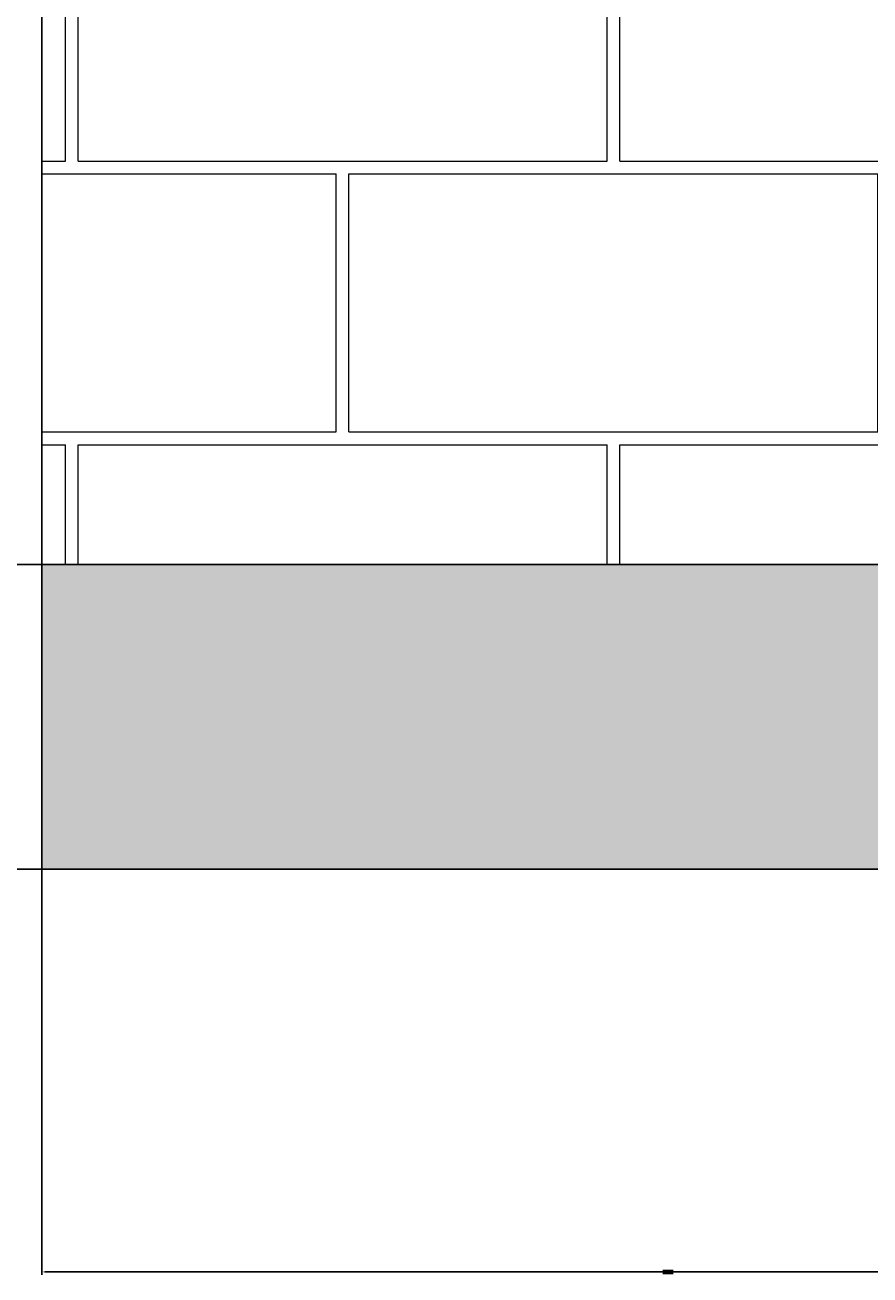
# Model space of a CAD drawing. Units: inches. Extents: x -128 to 854, y -395 to 398.
# Tile 52 of 61: x 417 to 467, y -395 to -322. Entities that reach past the tile are written whole.
import ezdxf

# ---------------------------------------------------------------- set-up
doc = ezdxf.new("R2010")
doc.units = ezdxf.units.IN
doc.header["$MEASUREMENT"] = 0
for name, color, linetype, lineweight in [('A-ANNO-DIMS', 2, 'Continuous', 18), ('A-ELEV', 3, 'Continuous', 25), ('A-ELEV-PATT', 8, 'Continuous', 13), ('C-GRAD', 7, 'Continuous', 25)]:
    doc.layers.add(name, color=color, linetype=linetype, lineweight=lineweight)
doc.styles.get("Standard").update_dxf_attribs({"font": 'arial.ttf'})
doc.dimstyles.get("Standard").update_dxf_attribs({"dimtxt": 0.18, "dimasz": 0.18, "dimexe": 0.18, "dimexo": 0.0625, "dimgap": 0.09, "dimtad": 0, "dimtih": 1, "dimtoh": 1, "dimdec": 1, "dimzin": 0, "dimdsep": 46, "dimlunit": 4, "dimtxsty": 'Standard', "dimcen": 0.09, "dimclrd": 1, "dimclre": 2, "dimclrt": 6, "dimadec": 0, "dimazin": 0, "dimtfac": 1, "dimtdec": 1, "dimtofl": 0, "dimtmove": 0, "dimatfit": 3, "dimfxl": 1, "dimtfill": 2, "dimtfillclr": 3, "dimtolj": 1, "dimtzin": 0, "dimarcsym": 0})

# ---------------------------------------------------------------- blocks, each defined once
blk = doc.blocks.new('*D134')
at = {"layer": 'A-ANNO-DIMS', "color": 2, "lineweight": -2, "transparency": 16777216}
for p, q in [((418.217, -191.476), (346.3, -191.476)), ((418.217, -371.476), (346.3, -371.476))]:
    blk.add_line(p, q, dxfattribs=at)
at = {"layer": 'A-ANNO-DIMS', "color": 1, "lineweight": -2, "transparency": 16777216}
for p, q in [((346.48, -191.656), (346.48, -281.295)), ((346.48, -371.296), (346.48, -281.658))]:
    blk.add_line(p, q, dxfattribs=at)
at = {"layer": 'A-ANNO-DIMS', "color": 1, "transparency": 16777216}
for points in [[(346.45, -191.656), (346.51, -191.656), (346.48, -191.476)], [(346.45, -371.296), (346.51, -371.296), (346.48, -371.476)]]:
    blk.add_solid(points, dxfattribs=at)
at = {"layer": 'Defpoints', "color": 0, "transparency": 16777216}
for p in [(346.48, -191.476), (418.28, -191.476), (418.28, -371.476)]:
    blk.add_point(p, dxfattribs=at)
at = {"layer": 'A-ANNO-DIMS', "color": 6, "transparency": 16777216, "insert": (346.48, -281.476), "char_height": 0.18, "attachment_point": 5, "bg_fill": 1, "box_fill_scale": 1.25, "bg_fill_color": 3, "bg_fill_transparency": 0}
blk.add_mtext('\\A1;15\'-0"', dxfattribs=at)
blk = doc.blocks.new('*D135')
at = {"layer": 'A-ANNO-DIMS', "color": 2, "lineweight": -2, "transparency": 16777216}
for p, q in [((418.28, -371.539), (418.28, -395.456)), ((492.252, -371.539), (492.252, -395.456))]:
    blk.add_line(p, q, dxfattribs=at)
at = {"layer": 'A-ANNO-DIMS', "color": 1, "lineweight": -2, "transparency": 16777216}
for p, q in [((418.46, -395.276), (454.936, -395.276)), ((492.072, -395.276), (455.596, -395.276))]:
    blk.add_line(p, q, dxfattribs=at)
at = {"layer": 'A-ANNO-DIMS', "color": 1, "transparency": 16777216}
for points in [[(418.46, -395.246), (418.46, -395.306), (418.28, -395.276)], [(492.072, -395.246), (492.072, -395.306), (492.252, -395.276)]]:
    blk.add_solid(points, dxfattribs=at)
at = {"layer": 'Defpoints', "color": 0, "transparency": 16777216}
for p in [(418.28, -371.476), (492.252, -371.476), (492.252, -395.276)]:
    blk.add_point(p, dxfattribs=at)
at = {"layer": 'A-ANNO-DIMS', "color": 6, "transparency": 16777216, "insert": (455.266, -395.276), "char_height": 0.18, "attachment_point": 5, "bg_fill": 1, "box_fill_scale": 1.25, "bg_fill_color": 3, "bg_fill_transparency": 0}
blk.add_mtext('\\A1;6\'-2"', dxfattribs=at)
blk = doc.blocks.new('*D140')
at = {"layer": 'A-ANNO-DIMS', "color": 2, "lineweight": -2, "transparency": 16777216}
for p, q in [((551.245, -257.476), (346.3, -257.476)), ((551.245, -353.476), (346.3, -353.476))]:
    blk.add_line(p, q, dxfattribs=at)
at = {"layer": 'A-ANNO-DIMS', "color": 1, "lineweight": -2, "transparency": 16777216}
for p, q in [((346.48, -257.656), (346.48, -305.295)), ((346.48, -353.296), (346.48, -305.658))]:
    blk.add_line(p, q, dxfattribs=at)
at = {"layer": 'A-ANNO-DIMS', "color": 1, "transparency": 16777216}
for points in [[(346.45, -257.656), (346.51, -257.656), (346.48, -257.476)], [(346.45, -353.296), (346.51, -353.296), (346.48, -353.476)]]:
    blk.add_solid(points, dxfattribs=at)
at = {"layer": 'Defpoints', "color": 0, "transparency": 16777216}
for p in [(346.48, -257.476), (551.307, -257.476), (551.307, -353.476)]:
    blk.add_point(p, dxfattribs=at)
at = {"layer": 'A-ANNO-DIMS', "color": 6, "transparency": 16777216, "insert": (346.48, -305.476), "char_height": 0.18, "attachment_point": 5, "bg_fill": 1, "box_fill_scale": 1.25, "bg_fill_color": 3, "bg_fill_transparency": 0}
blk.add_mtext('\\A1;8\'-0"', dxfattribs=at)

msp = doc.modelspace()

# ---------------------------------------------------------------- hatches: boundary and pattern name
at = {"layer": 'A-ELEV-PATT'}
h = msp.add_hatch(dxfattribs=at)
h.set_pattern_fill('AR-B816C', color=256, scale=2)
h.set_pattern_definition([(0, (468.407, -10.41), (16, 16), [31.25, -0.75]), (0, (452.407, -9.66), (16, 16), [31.25, -0.75]), (90, (468.407, -10.41), (-16, 16), [-16.75, 15.25]), (90, (467.657, -10.41), (-16, 16), [-16.75, 15.25])])
h.paths.add_polyline_path([(418.28, -353.476), (492.252, -353.476), (492.252, -257.476), (551.307, -257.476), (551.307, -353.476), (782.28, -353.476), (782.28, -233.476), (418.28, -233.476)])
h.paths.add_polyline_path([(668.28, -257.476), (730.28, -257.476), (730.28, -305.476), (668.28, -305.476)], flags=16)
h.paths.add_polyline_path([(673.28, -300.476), (673.28, -262.476), (725.28, -262.476), (725.28, -300.476)], flags=0)
h = msp.add_hatch(dxfattribs=at)
h.set_pattern_fill('AR-CONC', color=256, scale=2)
h.set_pattern_definition([(50, (468.407, -10.41), (14.3452, -1.25504), [1.5, -16.5]), (355, (468.407, -10.41), (-2.77503, 15.04384), [1.2, -13.2]), (100.4514, (469.602, -10.515), (11.57018, 13.7888), [1.2748, -14.02284]), (46.184, (468.407, -6.41), (21.3448, -3.3104), [2.25, -24.75]), (96.6356, (470.186, -6.686), (18.6932, 19.4824), [1.9122, -21.0343]), (351.184, (468.407, -6.41), (18.6932, 19.4824), [1.8, -19.8]), (21, (470.407, -7.41), (11.93814, -8.05238), [1.5, -16.5]), (326, (470.407, -7.41), (4.8663, 14.503), [1.2, -13.2]), (71.4514, (471.402, -8.081), (16.80445, 6.45062), [1.2748, -14.02284]), (37.5, (468.407, -10.4104), (0.243197, 6.657877), [0, -13.04, 0, -13.4, 0, -13.25]), (7.5, (468.407, -10.4104), (5.26139, 7.88823), [0, -7.64, 0, -12.74, 0, -5.05]), (327.5, (463.947, -10.4104), (10.67645, -0.4511), [0, -5, 0, -15.6, 0, -20.7]), (317.5, (461.947, -10.41), (11.66372, 2.0021), [0, -6.5, 0, -10.36, 0, -14.7])])
h.paths.add_polyline_path([(418.28, -353.476), (418.28, -371.476), (492.252, -371.476), (492.252, -353.476)])
h.paths.add_polyline_path([(782.28, -371.476), (782.28, -353.476), (551.307, -353.476), (551.307, -371.476)])

# ---------------------------------------------------------------- linework, layer by layer
at = {"layer": 'A-ELEV'}
for points in [[(418.28, -233.476), (782.28, -233.476), (782.28, -353.476), (418.28, -353.476)], [(418.28, -353.476), (782.28, -353.476), (782.28, -371.476), (418.28, -371.476)]]:
    msp.add_lwpolyline(points, close=True, dxfattribs=at)
at = {"layer": 'C-GRAD'}
msp.add_line((418.28, -371.476), (370.28, -371.476), dxfattribs=at)

# ---------------------------------------------------------------- dimensions: what is measured, and where the dimension line sits
at = {"layer": 'A-ANNO-DIMS'}
for base, p1, p2, picture, middle in [((346.48, -191.476), (418.28, -371.476), (418.28, -191.476), '*D134', (346.48, -281.476)), ((346.48, -257.476), (551.307, -353.476), (551.307, -257.476), '*D140', (346.48, -305.476))]:
    dim = msp.add_linear_dim(base=base, p1=p1, p2=p2, angle=90, dimstyle='Standard', override={"dimdec": 1, "dimlfac": 1, "dimrnd": 0, "dimzin": 1, "dimdsep": 46, "dimlunit": 4, "dimfrac": 2}, dxfattribs=at)
    dim.commit()
    dim.dimension.update_dxf_attribs({"geometry": picture, "text_midpoint": middle})
dim = msp.add_linear_dim(base=(492.252, -395.276), p1=(418.28, -371.476), p2=(492.252, -371.476), dimstyle='Standard', override={"dimdec": 1, "dimlfac": 1, "dimrnd": 0, "dimzin": 1, "dimdsep": 46, "dimlunit": 4, "dimfrac": 2}, dxfattribs=at)
dim.commit()
dim.dimension.update_dxf_attribs({"geometry": '*D135', "text_midpoint": (455.266, -395.276)})

doc.saveas('drawing.dxf')
